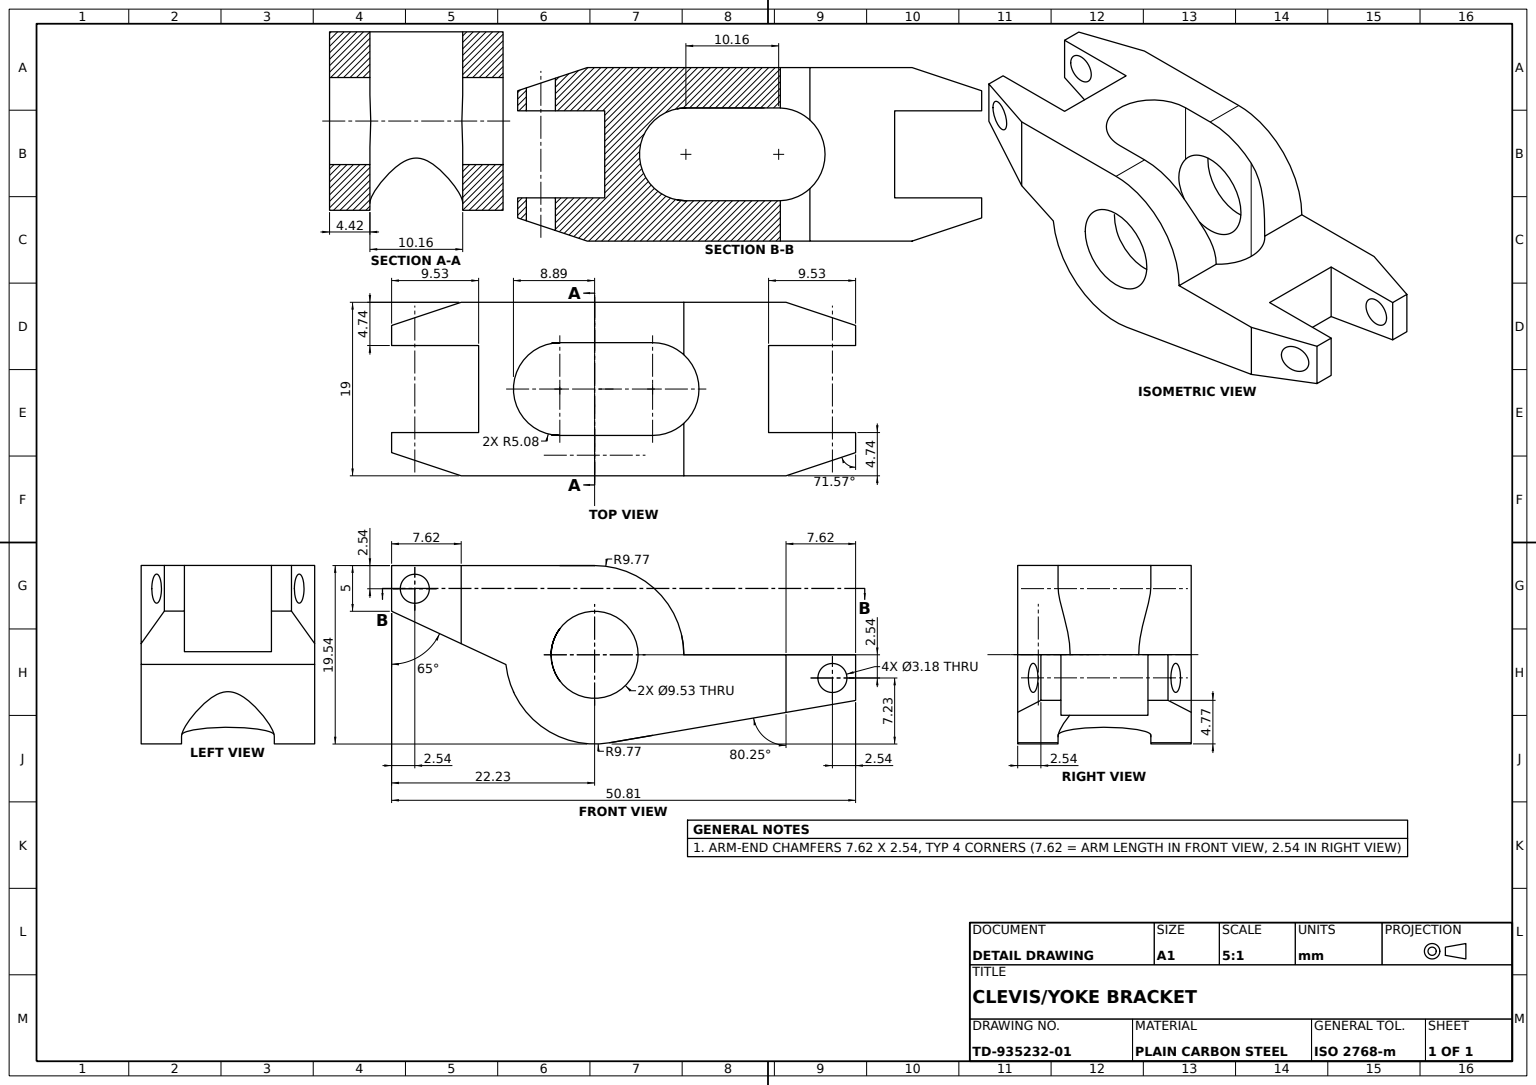
from build123d import *
from OCP.BRepFilletAPI import BRepFilletAPI_MakeChamfer

# Parameters (mm, degrees)
ROCKER_BODY_PROFILE_SKETCH_R      = 4.765
ROCKER_BODY_DEPTH                 = 9.5
ARM_END_CHAMFER_A_SIZE            = 7.62
ARM_END_CHAMFER_A_SIZE2           = 2.54
ARM_END_CHAMFER_B_SIZE            = 2.54
ARM_END_CHAMFER_B_SIZE2           = 7.62
FORK_SLOTS_SKETCH_W               = 9.53
FORK_SLOTS_SKETCH_H               = 9.53
FORK_SLOT_CUT_A_DEPTH             = 32.662585176
FORK_SLOT_CUT_B_DEPTH             = 32.662585176
FORK_SLOT_CUT_B_DEPTH_BACK        = 32.662585176
SKETCH2_2_W                       = 9.53
SKETCH2_2_H                       = 9.53
CENTRE_POCKET_DEPTH               = 32.662585176
CENTRE_POCKET_DEPTH_BACK          = 32.662585176
FORK_PIN_HOLES_2X_3_18_DEPTH      = 32.662585236
FORK_PIN_HOLES_2X_3_18_DEPTH_BACK = 32.662585236
FORK_PIN_HOLES_SKETCH_R           = 1.59


with BuildPart() as part:
    # Rocker Body Profile Sketch → Rocker Body (new, symmetric)
    with BuildSketch(Plane.XY):
        with BuildLine():
            Line((0, 9.77), (-22.23, 9.77))
            Line((-22.23, 9.77), (-22.23, 4.77))
            Line((-22.23, 4.77), (-9.711509246, -1.067468107))
            ThreePointArc((-9.711509246, -1.067468107), (-5.877874817, -7.804068659), (1.655323868, -9.628748771))
            Line((1.655323868, -9.628748771), (28.58, -5))
            Line((28.58, -5), (28.58, 0))
            Line((28.58, 0), (9.77, 0))
            ThreePointArc((9.77, 0), (6.908433252, 6.908433252), (0, 9.77))
        make_face()
        Circle(ROCKER_BODY_PROFILE_SKETCH_R, mode=Mode.SUBTRACT)
    extrude(amount=ROCKER_BODY_DEPTH, both=True)

    # Arm End Chamfer A
    arm_end_chamfer_a_edges = [part.edges().sort_by_distance(p)[0] for p in [
        (-22.23, 7.27, -9.5),
        (28.58, -2.5, -9.5),
    ]]
    arm_end_chamfer_a_side = [part.faces().sort_by_distance(p)[0] for p in [
        (-11.115, 9.225622585, -9.5),
    ]]
    chamfer(arm_end_chamfer_a_edges, length=ARM_END_CHAMFER_A_SIZE, length2=ARM_END_CHAMFER_A_SIZE2, reference=arm_end_chamfer_a_side[0])

    # Arm End Chamfer B: one chamfer whose edges measure the first distance from different faces: ONE call of the kernel's chamfer builder (chamfer() names one face for all edges)
    arm_end_chamfer_b_edges_1 = [part.edges().sort_by_distance(p)[0] for p in [
        (-22.23, 7.27, 9.5),
    ]]
    arm_end_chamfer_b_side_1 = [part.faces().sort_by_distance(p)[0] for p in [
        (-22.23, 7.27, 1.27),
    ]]
    arm_end_chamfer_b_edges_2 = [part.edges().sort_by_distance(p)[0] for p in [
        (28.58, -2.5, 9.5),
    ]]
    arm_end_chamfer_b_side_2 = [part.faces().sort_by_distance(p)[0] for p in [
        (28.58, -2.5, 1.27),
    ]]
    arm_end_chamfer_b = BRepFilletAPI_MakeChamfer(part.part.solid().wrapped)
    for e in arm_end_chamfer_b_edges_1:
        arm_end_chamfer_b.Add(ARM_END_CHAMFER_B_SIZE, ARM_END_CHAMFER_B_SIZE2, e.wrapped, arm_end_chamfer_b_side_1[0].wrapped)  # the first distance lies on this face
    for e in arm_end_chamfer_b_edges_2:
        arm_end_chamfer_b.Add(ARM_END_CHAMFER_B_SIZE, ARM_END_CHAMFER_B_SIZE2, e.wrapped, arm_end_chamfer_b_side_2[0].wrapped)  # the first distance lies on this face
    add(Compound.cast(arm_end_chamfer_b.Shape()), mode=Mode.REPLACE)

    # Fork Slots Sketch → Fork Slot Cut A (cut, through all)
    with BuildSketch(Plane(origin=(0, 0, 0), x_dir=(1, 0, 0), z_dir=(0, 1, 0))):
        with Locations((-17.465, 0)):
            Rectangle(FORK_SLOTS_SKETCH_W, FORK_SLOTS_SKETCH_H)
        with Locations((23.815, 0)):
            Rectangle(FORK_SLOTS_SKETCH_W, FORK_SLOTS_SKETCH_H)
    extrude(amount=-FORK_SLOT_CUT_A_DEPTH, mode=Mode.SUBTRACT)

    # Sketch2_2 → Fork Slot Cut B (cut, two sides: drawn at the far end of the back side and taken through both)
    with BuildSketch(Plane(origin=(0, 0, 0), x_dir=(1, 0, 0), z_dir=(0, 1, 0)).offset(-FORK_SLOT_CUT_B_DEPTH_BACK)):
        with Locations((-17.465, 0)):
            Rectangle(SKETCH2_2_W, SKETCH2_2_H)
        with Locations((23.815, 0)):
            Rectangle(SKETCH2_2_W, SKETCH2_2_H)
    extrude(amount=FORK_SLOT_CUT_B_DEPTH + FORK_SLOT_CUT_B_DEPTH_BACK, mode=Mode.SUBTRACT)

    # Centre Pocket Sketch → Centre Pocket (cut, two sides: drawn at the far end of the back side and taken through both)
    with BuildSketch(Plane(origin=(0, 0, 0), x_dir=(1, 0, 0), z_dir=(0, 1, 0)).offset(-CENTRE_POCKET_DEPTH_BACK)):
        with BuildLine():
            Line((-3.81, 5.08), (6.35, 5.08))
            ThreePointArc((6.35, 5.08), (11.43, 0), (6.35, -5.08))
            Line((6.35, -5.08), (-3.81, -5.08))
            ThreePointArc((-3.81, -5.08), (-8.89, 0), (-3.81, 5.08))
        make_face()
    extrude(amount=CENTRE_POCKET_DEPTH + CENTRE_POCKET_DEPTH_BACK, mode=Mode.SUBTRACT)

    # Fork Pin Holes Sketch → Fork Pin Holes 2x_3.18 (cut, two sides: drawn at the far end of the back side and taken through both)
    with BuildSketch(Plane.XY.offset(-FORK_PIN_HOLES_2X_3_18_DEPTH_BACK)):
        with Locations((-19.69, 7.23)):
            Circle(FORK_PIN_HOLES_SKETCH_R)
        with Locations((26.04, -2.54)):
            Circle(FORK_PIN_HOLES_SKETCH_R)
    extrude(amount=FORK_PIN_HOLES_2X_3_18_DEPTH + FORK_PIN_HOLES_2X_3_18_DEPTH_BACK, mode=Mode.SUBTRACT)


solid = part.part
